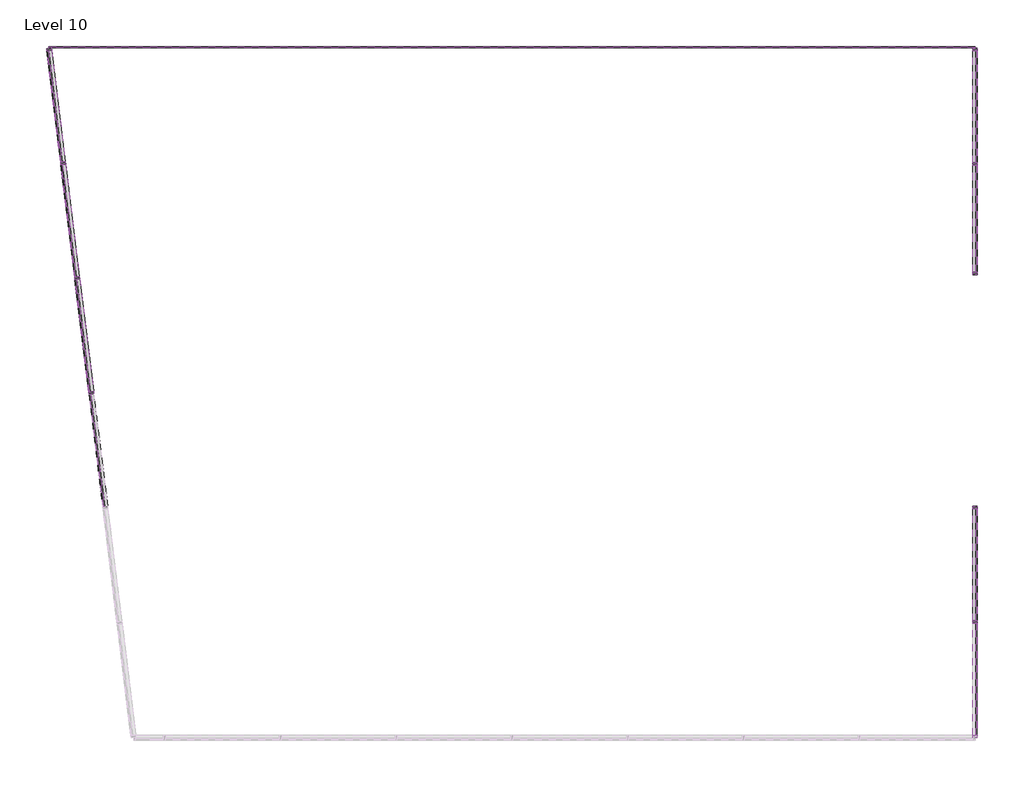
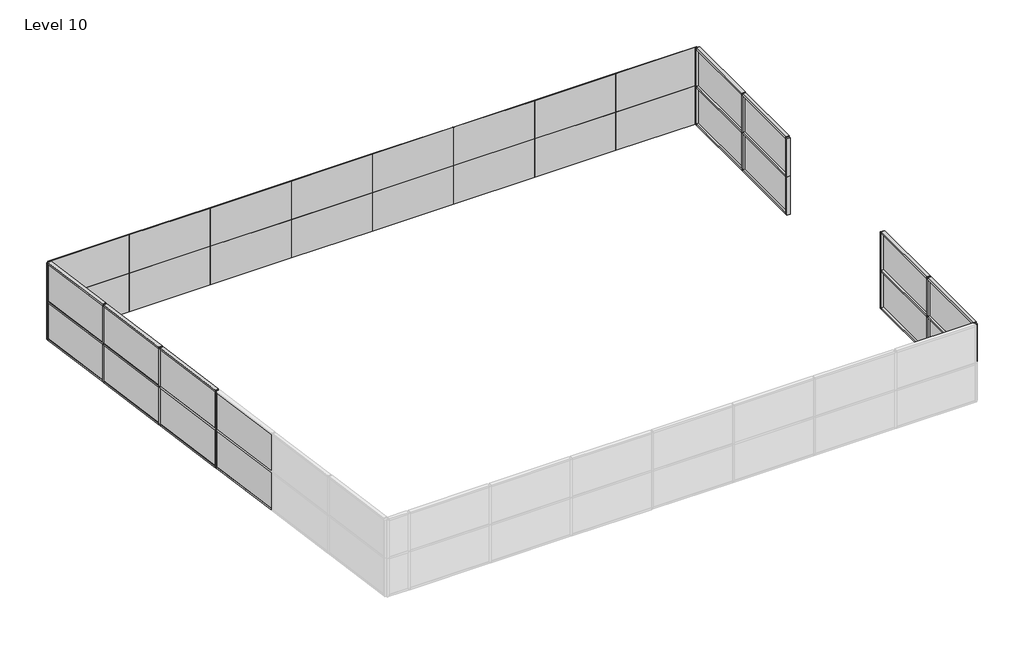
# One storey, part 2 of 2: 54 members, 40 plates.
"""IFC4 building model written with IfcOpenShell, lengths in millimetres."""

from ifc_helpers import new_model, si_unit, origin, place, context, project, spatial, transform, mapped, element, save
from components import member_71c27fd2, member_19d0a4ec, member_8cef0660, member_db480205, member_82905deb, member_4491d118, member_1b94d493, member_46bdb8c2, system_panel_glazed_1e57f9bb, system_panel_glazed_37f15d2e, system_panel_glazed_3620f98e, system_panel_glazed_e46d4b42, system_panel_glazed_2a6c68b7, system_panel_glazed_7fb1fc2b, system_panel_glazed_d483336f

model = new_model("IFC4")

# Units and contexts
model_context = context("Model", 3, world=origin())
ifc_project = project(units=[si_unit("LENGTHUNIT", "METRE", prefix="MILLI")], contexts=[model_context])

# Site, building, storey
site = spatial("IfcSite", under=ifc_project)
building = spatial("IfcBuilding", under=site)
storey = spatial("IfcBuildingStorey", under=building, Name="Level 10", Elevation=27432.0)

# Members
placement = place(None, origin())
member_shape = member_71c27fd2(model_context)
element("IfcMember", 1, ObjectType="Rectangular Mullion : 2.5\" x 5\" rectangular", at=placement, inside=storey, context=model_context, shape_type="MappedRepresentation", body=[
    mapped(member_shape, transform((-10473.7456604, 11109.5209701, 27432.0), x_axis=(0.0, 0.0, -1.0), y_axis=(-0.9925461516413222, -0.12186934340514599, 0.0), z_axis=(-0.12186934340514599, 0.9925461516413222, 0.0))),
])
element("IfcMember", 2, ObjectType="Rectangular Mullion : 2.5\" x 5\" rectangular", at=placement, inside=storey, context=model_context, shape_type="MappedRepresentation", body=[
    mapped(member_shape, transform((13902.5156363, -3899.3863708, 27432.0), x_axis=(0.0, 0.0, -1.0), y_axis=(1.0, 0.0, 0.0), z_axis=(0.0, -1.0, 0.0))),
])
element("IfcMember", 3, ObjectType="Rectangular Mullion : 2.5\" x 5\" rectangular", at=placement, inside=storey, context=model_context, shape_type="MappedRepresentation", body=[
    mapped(member_shape, transform((13902.5156363, 8156.2976505, 27432.0), x_axis=(0.0, 0.0, -1.0), y_axis=(1.0, 0.0, 0.0), z_axis=(0.0, -1.0, 0.0))),
])
member_2_shape = member_19d0a4ec(model_context)
element("IfcMember", 4, ObjectType="Rectangular Mullion : 2.5\" x 5\" rectangular", at=placement, inside=storey, context=model_context, shape_type="MappedRepresentation", body=[
    mapped(member_2_shape, transform((-10113.8959567, 8178.7803212, 28956.0), x_axis=(0.0, 0.0, 1.0), y_axis=(-0.9925461516413222, -0.12186934340514609, 0.0), z_axis=(0.12186934340514609, -0.9925461516413222, 0.0))),
])
element("IfcMember", 5, ObjectType="Rectangular Mullion : 2.5\" x 5\" rectangular", at=placement, inside=storey, context=model_context, shape_type="MappedRepresentation", body=[
    mapped(member_2_shape, transform((-10113.8959567, 8178.7803212, 30480.0), x_axis=(0.0, 0.0, 1.0), y_axis=(-0.9925461516413222, -0.12186934340514617, 0.0), z_axis=(0.12186934340514617, -0.9925461516413222, 0.0))),
])
element("IfcMember", 6, ObjectType="Rectangular Mullion : 2.5\" x 5\" rectangular", at=placement, inside=storey, context=model_context, shape_type="MappedRepresentation", body=[
    mapped(member_2_shape, transform((-10113.8959567, 8178.7803212, 28956.0), x_axis=(0.0, 0.0, 1.0), y_axis=(-0.9925461516413222, -0.12186934340514599, 0.0), z_axis=(0.12186934340514599, -0.9925461516413222, 0.0))),
])
element("IfcMember", 7, ObjectType="Rectangular Mullion : 2.5\" x 5\" rectangular", at=placement, inside=storey, context=model_context, shape_type="MappedRepresentation", body=[
    mapped(member_2_shape, transform((-10113.8959567, 8178.7803212, 30480.0), x_axis=(0.0, 0.0, 1.0), y_axis=(-0.9925461516413222, -0.12186934340514599, 0.0), z_axis=(0.12186934340514599, -0.9925461516413222, 0.0))),
])
element("IfcMember", 8, ObjectType="Rectangular Mullion : 2.5\" x 5\" rectangular", at=placement, inside=storey, context=model_context, shape_type="MappedRepresentation", body=[
    mapped(member_2_shape, transform((13902.5156363, -946.6363705, 28956.0), x_axis=(0.0, 0.0, 1.0), y_axis=(1.0, 0.0, 0.0), z_axis=(0.0, 1.0, 0.0))),
])
element("IfcMember", 9, ObjectType="Rectangular Mullion : 2.5\" x 5\" rectangular", at=placement, inside=storey, context=model_context, shape_type="MappedRepresentation", body=[
    mapped(member_2_shape, transform((13902.5156363, -3962.8863708, 28956.0), x_axis=(0.0, 0.0, 1.0), y_axis=(1.0, 0.0, 0.0), z_axis=(0.0, 1.0, 0.0))),
])
element("IfcMember", 10, ObjectType="Rectangular Mullion : 2.5\" x 5\" rectangular", at=placement, inside=storey, context=model_context, shape_type="MappedRepresentation", body=[
    mapped(member_2_shape, transform((13902.5156363, -946.6363705, 30480.0), x_axis=(0.0, 0.0, 1.0), y_axis=(1.0, 0.0, 0.0), z_axis=(0.0, 1.0, 0.0))),
])
element("IfcMember", 11, ObjectType="Rectangular Mullion : 2.5\" x 5\" rectangular", at=placement, inside=storey, context=model_context, shape_type="MappedRepresentation", body=[
    mapped(member_2_shape, transform((13902.5156363, -3962.8863708, 30480.0), x_axis=(0.0, 0.0, 1.0), y_axis=(1.0, 0.0, 0.0), z_axis=(0.0, 1.0, 0.0))),
])
element("IfcMember", 12, ObjectType="Rectangular Mullion : 2.5\" x 5\" rectangular", at=placement, inside=storey, context=model_context, shape_type="MappedRepresentation", body=[
    mapped(member_2_shape, transform((13902.5156363, 11109.0476508, 28956.0), x_axis=(0.0, 0.0, 1.0), y_axis=(1.0, 0.0, 0.0), z_axis=(0.0, 1.0, 0.0))),
])
element("IfcMember", 13, ObjectType="Rectangular Mullion : 2.5\" x 5\" rectangular", at=placement, inside=storey, context=model_context, shape_type="MappedRepresentation", body=[
    mapped(member_2_shape, transform((13902.5156363, 11109.0476508, 30480.0), x_axis=(0.0, 0.0, 1.0), y_axis=(1.0, 0.0, 0.0), z_axis=(0.0, 1.0, 0.0))),
])
member_3_shape = member_8cef0660(model_context)
element("IfcMember", 14, ObjectType="Rectangular Mullion : 2.5\" x 5\" rectangular", at=placement, inside=storey, context=model_context, shape_type="MappedRepresentation", body=[
    mapped(member_3_shape, transform((-9370.9804393, 2128.2189808, 28956.0), x_axis=(0.0, 0.0, 1.0), y_axis=(-0.9925461516413223, -0.12186934340514563, 0.0), z_axis=(0.12186934340514562, -0.9925461516413222, 0.0))),
])
element("IfcMember", 15, ObjectType="Rectangular Mullion : 2.5\" x 5\" rectangular", at=placement, inside=storey, context=model_context, shape_type="MappedRepresentation", body=[
    mapped(member_3_shape, transform((-9742.438198, 5153.499651, 28956.0), x_axis=(0.0, 0.0, 1.0), y_axis=(-0.9925461516413222, -0.12186934340514602, 0.0), z_axis=(0.12186934340514602, -0.9925461516413222, 0.0))),
])
element("IfcMember", 16, ObjectType="Rectangular Mullion : 2.5\" x 5\" rectangular", at=placement, inside=storey, context=model_context, shape_type="MappedRepresentation", body=[
    mapped(member_3_shape, transform((-9370.9804393, 2128.2189808, 30480.0), x_axis=(0.0, 0.0, 1.0), y_axis=(-0.9925461516413222, -0.12186934340514592, 0.0), z_axis=(0.12186934340514592, -0.9925461516413222, 0.0))),
])
element("IfcMember", 17, ObjectType="Rectangular Mullion : 2.5\" x 5\" rectangular", at=placement, inside=storey, context=model_context, shape_type="MappedRepresentation", body=[
    mapped(member_3_shape, transform((-9742.438198, 5153.499651, 30480.0), x_axis=(0.0, 0.0, 1.0), y_axis=(-0.9925461516413222, -0.1218693434051457, 0.0), z_axis=(0.1218693434051457, -0.9925461516413222, 0.0))),
])
element("IfcMember", 18, ObjectType="Rectangular Mullion : 2.5\" x 5\" rectangular", at=placement, inside=storey, context=model_context, shape_type="MappedRepresentation", body=[
    mapped(member_3_shape, transform((-9370.9804393, 2128.2189808, 28956.0), x_axis=(0.0, 0.0, 1.0), y_axis=(-0.9925461516413222, -0.12186934340514592, 0.0), z_axis=(0.12186934340514592, -0.9925461516413222, 0.0))),
])
element("IfcMember", 19, ObjectType="Rectangular Mullion : 2.5\" x 5\" rectangular", at=placement, inside=storey, context=model_context, shape_type="MappedRepresentation", body=[
    mapped(member_3_shape, transform((-9742.438198, 5153.499651, 28956.0), x_axis=(0.0, 0.0, 1.0), y_axis=(-0.9925461516413222, -0.1218693434051457, 0.0), z_axis=(0.1218693434051457, -0.9925461516413222, 0.0))),
])
element("IfcMember", 20, ObjectType="Rectangular Mullion : 2.5\" x 5\" rectangular", at=placement, inside=storey, context=model_context, shape_type="MappedRepresentation", body=[
    mapped(member_3_shape, transform((-9370.9804393, 2128.2189808, 30480.0), x_axis=(0.0, 0.0, 1.0), y_axis=(-0.9925461516413222, -0.12186934340514595, 0.0), z_axis=(0.12186934340514595, -0.9925461516413222, 0.0))),
])
element("IfcMember", 21, ObjectType="Rectangular Mullion : 2.5\" x 5\" rectangular", at=placement, inside=storey, context=model_context, shape_type="MappedRepresentation", body=[
    mapped(member_3_shape, transform((-9742.438198, 5153.499651, 30480.0), x_axis=(0.0, 0.0, 1.0), y_axis=(-0.9925461516413222, -0.12186934340514606, 0.0), z_axis=(0.12186934340514606, -0.9925461516413222, 0.0))),
])
member_4_shape = member_db480205(model_context)
element("IfcMember", 22, ObjectType="Rectangular Mullion : 2.5\" x 5\" rectangular", at=placement, inside=storey, context=model_context, shape_type="MappedRepresentation", body=[
    mapped(member_4_shape, transform((-9363.241736, 2065.1923001, 27432.0), x_axis=(0.0, 0.0, -1.0), y_axis=(-0.9925461516413223, -0.12186934340514559, 0.0), z_axis=(-0.12186934340514559, 0.9925461516413223, 0.0))),
])
element("IfcMember", 23, ObjectType="Rectangular Mullion : 2.5\" x 5\" rectangular", at=placement, inside=storey, context=model_context, shape_type="MappedRepresentation", body=[
    mapped(member_4_shape, transform((-9734.6994947, 5090.4729703, 27432.0), x_axis=(0.0, 0.0, -1.0), y_axis=(-0.9925461516413222, -0.12186934340514592, 0.0), z_axis=(-0.12186934340514592, 0.9925461516413222, 0.0))),
])
element("IfcMember", 24, ObjectType="Rectangular Mullion : 2.5\" x 5\" rectangular", at=placement, inside=storey, context=model_context, shape_type="MappedRepresentation", body=[
    mapped(member_4_shape, transform((-10106.1572534, 8115.7536405, 27432.0), x_axis=(0.0, 0.0, -1.0), y_axis=(-0.9925461516413222, -0.12186934340514606, 0.0), z_axis=(-0.12186934340514606, 0.9925461516413222, 0.0))),
])
member_5_shape = member_82905deb(model_context)
element("IfcMember", 25, ObjectType="Rectangular Mullion : 2.5\" x 5\" rectangular", at=placement, inside=storey, context=model_context, shape_type="MappedRepresentation", body=[
    mapped(member_5_shape, transform((-9367.1110876, 2096.7056405, 28956.0), x_axis=(-0.1218693434051459, 0.9925461516413222, 0.0), y_axis=(-0.9925461516413222, -0.1218693434051459, 0.0), z_axis=(0.0, 0.0, 1.0))),
])
element("IfcMember", 26, ObjectType="Rectangular Mullion : 2.5\" x 5\" rectangular", at=placement, inside=storey, context=model_context, shape_type="MappedRepresentation", body=[
    mapped(member_5_shape, transform((-9738.5688463, 5121.9863107, 28956.0), x_axis=(-0.1218693434051459, 0.9925461516413222, 0.0), y_axis=(-0.9925461516413222, -0.1218693434051459, 0.0), z_axis=(0.0, 0.0, 1.0))),
])
element("IfcMember", 27, ObjectType="Rectangular Mullion : 2.5\" x 5\" rectangular", at=placement, inside=storey, context=model_context, shape_type="MappedRepresentation", body=[
    mapped(member_5_shape, transform((-10110.026605, 8147.2669809, 28956.0), x_axis=(-0.1218693434051459, 0.9925461516413222, 0.0), y_axis=(-0.9925461516413222, -0.1218693434051459, 0.0), z_axis=(0.0, 0.0, 1.0))),
])
element("IfcMember", 28, ObjectType="Rectangular Mullion : 2.5\" x 5\" rectangular", at=placement, inside=storey, context=model_context, shape_type="MappedRepresentation", body=[
    mapped(member_5_shape, transform((13902.5156363, -3931.1363708, 28956.0), x_axis=(0.0, -1.0, 0.0), y_axis=(1.0, 0.0, 0.0), z_axis=(0.0, 0.0, 1.0))),
])
element("IfcMember", 29, ObjectType="Rectangular Mullion : 2.5\" x 5\" rectangular", at=placement, inside=storey, context=model_context, shape_type="MappedRepresentation", body=[
    mapped(member_5_shape, transform((13902.5156363, 8124.5476505, 28956.0), x_axis=(0.0, -1.0, 0.0), y_axis=(1.0, 0.0, 0.0), z_axis=(0.0, 0.0, 1.0))),
])
element("IfcMember", 30, ObjectType="Rectangular Mullion : 2.5\" x 5\" rectangular", at=placement, inside=storey, context=model_context, shape_type="MappedRepresentation", body=[
    mapped(member_5_shape, transform((-9367.1110876, 2096.7056405, 28956.0), x_axis=(-0.1218693434051459, 0.9925461516413222, 0.0), y_axis=(-0.9925461516413222, -0.1218693434051459, 0.0), z_axis=(0.0, 0.0, 1.0))),
])
element("IfcMember", 31, ObjectType="Rectangular Mullion : 2.5\" x 5\" rectangular", at=placement, inside=storey, context=model_context, shape_type="MappedRepresentation", body=[
    mapped(member_5_shape, transform((-9367.1110876, 2096.7056405, 30480.0), x_axis=(-0.1218693434051459, 0.9925461516413222, 0.0), y_axis=(-0.9925461516413222, -0.1218693434051459, 0.0), z_axis=(0.0, 0.0, 1.0))),
])
element("IfcMember", 32, ObjectType="Rectangular Mullion : 2.5\" x 5\" rectangular", at=placement, inside=storey, context=model_context, shape_type="MappedRepresentation", body=[
    mapped(member_5_shape, transform((-9738.5688463, 5121.9863107, 28956.0), x_axis=(-0.1218693434051459, 0.9925461516413222, 0.0), y_axis=(-0.9925461516413222, -0.1218693434051459, 0.0), z_axis=(0.0, 0.0, 1.0))),
])
element("IfcMember", 33, ObjectType="Rectangular Mullion : 2.5\" x 5\" rectangular", at=placement, inside=storey, context=model_context, shape_type="MappedRepresentation", body=[
    mapped(member_5_shape, transform((-9738.5688463, 5121.9863107, 30480.0), x_axis=(-0.1218693434051459, 0.9925461516413222, 0.0), y_axis=(-0.9925461516413222, -0.1218693434051459, 0.0), z_axis=(0.0, 0.0, 1.0))),
])
element("IfcMember", 34, ObjectType="Rectangular Mullion : 2.5\" x 5\" rectangular", at=placement, inside=storey, context=model_context, shape_type="MappedRepresentation", body=[
    mapped(member_5_shape, transform((-10110.026605, 8147.2669809, 28956.0), x_axis=(-0.1218693434051459, 0.9925461516413222, 0.0), y_axis=(-0.9925461516413222, -0.1218693434051459, 0.0), z_axis=(0.0, 0.0, 1.0))),
])
element("IfcMember", 35, ObjectType="Rectangular Mullion : 2.5\" x 5\" rectangular", at=placement, inside=storey, context=model_context, shape_type="MappedRepresentation", body=[
    mapped(member_5_shape, transform((-10110.026605, 8147.2669809, 30480.0), x_axis=(-0.1218693434051459, 0.9925461516413222, 0.0), y_axis=(-0.9925461516413222, -0.1218693434051459, 0.0), z_axis=(0.0, 0.0, 1.0))),
])
element("IfcMember", 36, ObjectType="Rectangular Mullion : 2.5\" x 5\" rectangular", at=placement, inside=storey, context=model_context, shape_type="MappedRepresentation", body=[
    mapped(member_5_shape, transform((-9367.1110876, 2096.7056405, 30480.0), x_axis=(-0.1218693434051459, 0.9925461516413222, 0.0), y_axis=(-0.9925461516413222, -0.1218693434051459, 0.0), z_axis=(0.0, 0.0, 1.0))),
])
element("IfcMember", 37, ObjectType="Rectangular Mullion : 2.5\" x 5\" rectangular", at=placement, inside=storey, context=model_context, shape_type="MappedRepresentation", body=[
    mapped(member_5_shape, transform((-9738.5688463, 5121.9863107, 30480.0), x_axis=(-0.1218693434051459, 0.9925461516413222, 0.0), y_axis=(-0.9925461516413222, -0.1218693434051459, 0.0), z_axis=(0.0, 0.0, 1.0))),
])
element("IfcMember", 38, ObjectType="Rectangular Mullion : 2.5\" x 5\" rectangular", at=placement, inside=storey, context=model_context, shape_type="MappedRepresentation", body=[
    mapped(member_5_shape, transform((-10110.026605, 8147.2669809, 30480.0), x_axis=(-0.1218693434051459, 0.9925461516413222, 0.0), y_axis=(-0.9925461516413222, -0.1218693434051459, 0.0), z_axis=(0.0, 0.0, 1.0))),
])
element("IfcMember", 39, ObjectType="Rectangular Mullion : 2.5\" x 5\" rectangular", at=placement, inside=storey, context=model_context, shape_type="MappedRepresentation", body=[
    mapped(member_5_shape, transform((13902.5156363, -3931.1363708, 30480.0), x_axis=(0.0, -1.0, 0.0), y_axis=(1.0, 0.0, 0.0), z_axis=(0.0, 0.0, 1.0))),
])
element("IfcMember", 40, ObjectType="Rectangular Mullion : 2.5\" x 5\" rectangular", at=placement, inside=storey, context=model_context, shape_type="MappedRepresentation", body=[
    mapped(member_5_shape, transform((13902.5156363, 8124.5476505, 30480.0), x_axis=(0.0, -1.0, 0.0), y_axis=(1.0, 0.0, 0.0), z_axis=(0.0, 0.0, 1.0))),
])
member_6_shape = member_4491d118(model_context)
element("IfcMember", 41, ObjectType="Rectangular Mullion : 2.5\" x 5\" rectangular", at=placement, inside=storey, context=model_context, shape_type="MappedRepresentation", body=[
    mapped(member_6_shape, transform((13902.5156363, -883.1363705, 27432.0), x_axis=(0.0, 1.0, 0.0), y_axis=(1.0, 0.0, 0.0), z_axis=(0.0, 0.0, -1.0))),
])
element("IfcMember", 42, ObjectType="Rectangular Mullion : 2.5\" x 5\" rectangular", at=placement, inside=storey, context=model_context, shape_type="MappedRepresentation", body=[
    mapped(member_6_shape, transform((13902.5156363, 11172.5476508, 27432.0), x_axis=(0.0, 1.0, 0.0), y_axis=(1.0, 0.0, 0.0), z_axis=(0.0, 0.0, -1.0))),
])
element("IfcMember", 43, ObjectType="Rectangular Mullion : 2.5\" x 5\" rectangular", at=placement, inside=storey, context=model_context, shape_type="MappedRepresentation", body=[
    mapped(member_6_shape, transform((13902.5156363, -883.1363705, 28956.0), x_axis=(0.0, 1.0, 0.0), y_axis=(1.0, 0.0, 0.0), z_axis=(0.0, 0.0, -1.0))),
])
element("IfcMember", 44, ObjectType="Rectangular Mullion : 2.5\" x 5\" rectangular", at=placement, inside=storey, context=model_context, shape_type="MappedRepresentation", body=[
    mapped(member_6_shape, transform((13902.5156363, 11172.5476508, 28956.0), x_axis=(0.0, 1.0, 0.0), y_axis=(1.0, 0.0, 0.0), z_axis=(0.0, 0.0, -1.0))),
])
element("IfcMember", 45, ObjectType="Rectangular Mullion : 2.5\" x 5\" rectangular", at=placement, inside=storey, context=model_context, shape_type="MappedRepresentation", body=[
    mapped(member_6_shape, transform((-10481.4843637, 11172.5476508, 28956.0), x_axis=(-0.1218693434051459, 0.9925461516413222, 0.0), y_axis=(-0.9925461516413222, -0.1218693434051459, 0.0), z_axis=(0.0, 0.0, 1.0))),
])
element("IfcMember", 46, ObjectType="Rectangular Mullion : 2.5\" x 5\" rectangular", at=placement, inside=storey, context=model_context, shape_type="MappedRepresentation", body=[
    mapped(member_6_shape, transform((13902.5156363, 5212.8636295, 28956.0), x_axis=(0.0, -1.0, 0.0), y_axis=(1.0, 0.0, 0.0), z_axis=(0.0, 0.0, 1.0))),
])
element("IfcMember", 47, ObjectType="Rectangular Mullion : 2.5\" x 5\" rectangular", at=placement, inside=storey, context=model_context, shape_type="MappedRepresentation", body=[
    mapped(member_6_shape, transform((-10481.4843637, 11172.5476508, 28956.0), x_axis=(-0.1218693434051459, 0.9925461516413222, 0.0), y_axis=(-0.9925461516413222, -0.1218693434051459, 0.0), z_axis=(0.0, 0.0, 1.0))),
])
element("IfcMember", 48, ObjectType="Rectangular Mullion : 2.5\" x 5\" rectangular", at=placement, inside=storey, context=model_context, shape_type="MappedRepresentation", body=[
    mapped(member_6_shape, transform((-10481.4843637, 11172.5476508, 30480.0), x_axis=(-0.1218693434051459, 0.9925461516413222, 0.0), y_axis=(-0.9925461516413222, -0.1218693434051459, 0.0), z_axis=(0.0, 0.0, 1.0))),
])
element("IfcMember", 49, ObjectType="Rectangular Mullion : 2.5\" x 5\" rectangular", at=placement, inside=storey, context=model_context, shape_type="MappedRepresentation", body=[
    mapped(member_6_shape, transform((-10481.4843637, 11172.5476508, 30480.0), x_axis=(-0.1218693434051459, 0.9925461516413222, 0.0), y_axis=(-0.9925461516413222, -0.1218693434051459, 0.0), z_axis=(0.0, 0.0, 1.0))),
])
element("IfcMember", 50, ObjectType="Rectangular Mullion : 2.5\" x 5\" rectangular", at=placement, inside=storey, context=model_context, shape_type="MappedRepresentation", body=[
    mapped(member_6_shape, transform((13902.5156363, -6979.1363705, 30480.0), x_axis=(0.0, -1.0, 0.0), y_axis=(1.0, 0.0, 0.0), z_axis=(0.0, 0.0, 1.0))),
])
element("IfcMember", 51, ObjectType="Rectangular Mullion : 2.5\" x 5\" rectangular", at=placement, inside=storey, context=model_context, shape_type="MappedRepresentation", body=[
    mapped(member_6_shape, transform((13902.5156363, 5212.8636295, 30480.0), x_axis=(0.0, -1.0, 0.0), y_axis=(1.0, 0.0, 0.0), z_axis=(0.0, 0.0, 1.0))),
])
member_7_shape = member_1b94d493(model_context)
element("IfcMember", 52, ObjectType="Rectangular Mullion : 2.5\" x 5\" rectangular", at=placement, inside=storey, context=model_context, shape_type="MappedRepresentation", body=[
    mapped(member_7_shape, transform((13902.5156363, 5276.3636295, 27432.0), x_axis=(0.0, 0.0, -1.0), y_axis=(1.0, 0.0, 0.0), z_axis=(0.0, -1.0, 0.0))),
])
member_8_shape = member_46bdb8c2(model_context)
element("IfcMember", 53, ObjectType="Rectangular Mullion : 2.5\" x 5\" rectangular", at=placement, inside=storey, context=model_context, shape_type="MappedRepresentation", body=[
    mapped(member_8_shape, transform((13902.5156363, 8092.7976505, 28956.0), x_axis=(0.0, 0.0, 1.0), y_axis=(1.0, 0.0, 0.0), z_axis=(0.0, 1.0, 0.0))),
])
element("IfcMember", 54, ObjectType="Rectangular Mullion : 2.5\" x 5\" rectangular", at=placement, inside=storey, context=model_context, shape_type="MappedRepresentation", body=[
    mapped(member_8_shape, transform((13902.5156363, 8092.7976505, 30480.0), x_axis=(0.0, 0.0, 1.0), y_axis=(1.0, 0.0, 0.0), z_axis=(0.0, 1.0, 0.0))),
])

# Plates
system_panel_glazed_shape = system_panel_glazed_1e57f9bb(model_context)
element("IfcPlate", 55, ObjectType="System Panel : Glazed", at=placement, inside=storey, context=model_context, shape_type="MappedRepresentation", body=[
    mapped(system_panel_glazed_shape, transform((-8957.4843636, 11172.5476508, 27432.0), x_axis=(1.0, 0.0, 0.0), y_axis=(0.0, 1.0, 0.0), z_axis=(0.0, 0.0, 1.0))),
])
element("IfcPlate", 56, ObjectType="System Panel : Glazed", at=placement, inside=storey, context=model_context, shape_type="MappedRepresentation", body=[
    mapped(system_panel_glazed_shape, transform((-5909.4843634, 11172.5476508, 27432.0), x_axis=(1.0, 0.0, 0.0), y_axis=(0.0, 1.0, 0.0), z_axis=(0.0, 0.0, 1.0))),
])
element("IfcPlate", 57, ObjectType="System Panel : Glazed", at=placement, inside=storey, context=model_context, shape_type="MappedRepresentation", body=[
    mapped(system_panel_glazed_shape, transform((-2861.4843634, 11172.5476508, 27432.0), x_axis=(1.0, 0.0, 0.0), y_axis=(0.0, 1.0, 0.0), z_axis=(0.0, 0.0, 1.0))),
])
element("IfcPlate", 58, ObjectType="System Panel : Glazed", at=placement, inside=storey, context=model_context, shape_type="MappedRepresentation", body=[
    mapped(system_panel_glazed_shape, transform((186.5156366, 11172.5476508, 27432.0), x_axis=(1.0, 0.0, 0.0), y_axis=(0.0, 1.0, 0.0), z_axis=(0.0, 0.0, 1.0))),
])
element("IfcPlate", 59, ObjectType="System Panel : Glazed", at=placement, inside=storey, context=model_context, shape_type="MappedRepresentation", body=[
    mapped(system_panel_glazed_shape, transform((3234.5156366, 11172.5476508, 27432.0), x_axis=(1.0, 0.0, 0.0), y_axis=(0.0, 1.0, 0.0), z_axis=(0.0, 0.0, 1.0))),
])
element("IfcPlate", 60, ObjectType="System Panel : Glazed", at=placement, inside=storey, context=model_context, shape_type="MappedRepresentation", body=[
    mapped(system_panel_glazed_shape, transform((6282.5156366, 11172.5476508, 27432.0), x_axis=(1.0, 0.0, 0.0), y_axis=(0.0, 1.0, 0.0), z_axis=(0.0, 0.0, 1.0))),
])
element("IfcPlate", 61, ObjectType="System Panel : Glazed", at=placement, inside=storey, context=model_context, shape_type="MappedRepresentation", body=[
    mapped(system_panel_glazed_shape, transform((9330.5156366, 11172.5476508, 27432.0), x_axis=(1.0, 0.0, 0.0), y_axis=(0.0, 1.0, 0.0), z_axis=(0.0, 0.0, 1.0))),
])
element("IfcPlate", 62, ObjectType="System Panel : Glazed", at=placement, inside=storey, context=model_context, shape_type="MappedRepresentation", body=[
    mapped(system_panel_glazed_shape, transform((12378.5156364, 11172.5476508, 27432.0), x_axis=(1.0, 0.0, 0.0), y_axis=(0.0, 1.0, 0.0), z_axis=(0.0, 0.0, 1.0))),
])
element("IfcPlate", 63, ObjectType="System Panel : Glazed", at=placement, inside=storey, context=model_context, shape_type="MappedRepresentation", body=[
    mapped(system_panel_glazed_shape, transform((-8957.4843636, 11172.5476508, 28956.0), x_axis=(1.0, 0.0, 0.0), y_axis=(0.0, 1.0, 0.0), z_axis=(0.0, 0.0, 1.0))),
])
element("IfcPlate", 64, ObjectType="System Panel : Glazed", at=placement, inside=storey, context=model_context, shape_type="MappedRepresentation", body=[
    mapped(system_panel_glazed_shape, transform((-5909.4843634, 11172.5476508, 28956.0), x_axis=(1.0, 0.0, 0.0), y_axis=(0.0, 1.0, 0.0), z_axis=(0.0, 0.0, 1.0))),
])
element("IfcPlate", 65, ObjectType="System Panel : Glazed", at=placement, inside=storey, context=model_context, shape_type="MappedRepresentation", body=[
    mapped(system_panel_glazed_shape, transform((-2861.4843634, 11172.5476508, 28956.0), x_axis=(1.0, 0.0, 0.0), y_axis=(0.0, 1.0, 0.0), z_axis=(0.0, 0.0, 1.0))),
])
element("IfcPlate", 66, ObjectType="System Panel : Glazed", at=placement, inside=storey, context=model_context, shape_type="MappedRepresentation", body=[
    mapped(system_panel_glazed_shape, transform((186.5156366, 11172.5476508, 28956.0), x_axis=(1.0, 0.0, 0.0), y_axis=(0.0, 1.0, 0.0), z_axis=(0.0, 0.0, 1.0))),
])
element("IfcPlate", 67, ObjectType="System Panel : Glazed", at=placement, inside=storey, context=model_context, shape_type="MappedRepresentation", body=[
    mapped(system_panel_glazed_shape, transform((3234.5156366, 11172.5476508, 28956.0), x_axis=(1.0, 0.0, 0.0), y_axis=(0.0, 1.0, 0.0), z_axis=(0.0, 0.0, 1.0))),
])
element("IfcPlate", 68, ObjectType="System Panel : Glazed", at=placement, inside=storey, context=model_context, shape_type="MappedRepresentation", body=[
    mapped(system_panel_glazed_shape, transform((6282.5156366, 11172.5476508, 28956.0), x_axis=(1.0, 0.0, 0.0), y_axis=(0.0, 1.0, 0.0), z_axis=(0.0, 0.0, 1.0))),
])
element("IfcPlate", 69, ObjectType="System Panel : Glazed", at=placement, inside=storey, context=model_context, shape_type="MappedRepresentation", body=[
    mapped(system_panel_glazed_shape, transform((9330.5156366, 11172.5476508, 28956.0), x_axis=(1.0, 0.0, 0.0), y_axis=(0.0, 1.0, 0.0), z_axis=(0.0, 0.0, 1.0))),
])
element("IfcPlate", 70, ObjectType="System Panel : Glazed", at=placement, inside=storey, context=model_context, shape_type="MappedRepresentation", body=[
    mapped(system_panel_glazed_shape, transform((12378.5156364, 11172.5476508, 28956.0), x_axis=(1.0, 0.0, 0.0), y_axis=(0.0, 1.0, 0.0), z_axis=(0.0, 0.0, 1.0))),
])
system_panel_glazed_2_shape = system_panel_glazed_37f15d2e(model_context)
element("IfcPlate", 71, ObjectType="System Panel : Glazed", at=placement, inside=storey, context=model_context, shape_type="MappedRepresentation", body=[
    mapped(system_panel_glazed_2_shape, transform((13902.5156363, -2423.0113706, 27495.5), x_axis=(0.0, -1.0, 0.0), y_axis=(1.0, 0.0, 0.0), z_axis=(0.0, 0.0, 1.0))),
])
element("IfcPlate", 72, ObjectType="System Panel : Glazed", at=placement, inside=storey, context=model_context, shape_type="MappedRepresentation", body=[
    mapped(system_panel_glazed_2_shape, transform((13902.5156363, 9632.6726506, 27495.5), x_axis=(0.0, -1.0, 0.0), y_axis=(1.0, 0.0, 0.0), z_axis=(0.0, 0.0, 1.0))),
])
element("IfcPlate", 73, ObjectType="System Panel : Glazed", at=placement, inside=storey, context=model_context, shape_type="MappedRepresentation", body=[
    mapped(system_panel_glazed_2_shape, transform((-10293.8208085, 9644.1506457, 27495.5), x_axis=(-0.1218693434051459, 0.9925461516413222, 0.0), y_axis=(-0.9925461516413222, -0.1218693434051459, 0.0), z_axis=(0.0, 0.0, 1.0))),
])
element("IfcPlate", 74, ObjectType="System Panel : Glazed", at=placement, inside=storey, context=model_context, shape_type="MappedRepresentation", body=[
    mapped(system_panel_glazed_2_shape, transform((13902.5156363, -5439.2613706, 27495.5), x_axis=(0.0, -1.0, 0.0), y_axis=(1.0, 0.0, 0.0), z_axis=(0.0, 0.0, 1.0))),
])
system_panel_glazed_3_shape = system_panel_glazed_3620f98e(model_context)
element("IfcPlate", 75, ObjectType="System Panel : Glazed", at=placement, inside=storey, context=model_context, shape_type="MappedRepresentation", body=[
    mapped(system_panel_glazed_3_shape, transform((-9181.3822083, 584.0653054, 27495.5), x_axis=(-0.1218693434051459, 0.9925461516413222, 0.0), y_axis=(-0.9925461516413222, -0.1218693434051459, 0.0), z_axis=(0.0, 0.0, 1.0))),
])
element("IfcPlate", 76, ObjectType="System Panel : Glazed", at=placement, inside=storey, context=model_context, shape_type="MappedRepresentation", body=[
    mapped(system_panel_glazed_3_shape, transform((-9552.839967, 3609.3459756, 27495.5), x_axis=(-0.1218693434051459, 0.9925461516413222, 0.0), y_axis=(-0.9925461516413222, -0.1218693434051459, 0.0), z_axis=(0.0, 0.0, 1.0))),
])
element("IfcPlate", 77, ObjectType="System Panel : Glazed", at=placement, inside=storey, context=model_context, shape_type="MappedRepresentation", body=[
    mapped(system_panel_glazed_3_shape, transform((-9924.2977257, 6634.6266458, 27495.5), x_axis=(-0.1218693434051459, 0.9925461516413222, 0.0), y_axis=(-0.9925461516413222, -0.1218693434051459, 0.0), z_axis=(0.0, 0.0, 1.0))),
])
system_panel_glazed_4_shape = system_panel_glazed_e46d4b42(model_context)
element("IfcPlate", 78, ObjectType="System Panel : Glazed", at=placement, inside=storey, context=model_context, shape_type="MappedRepresentation", body=[
    mapped(system_panel_glazed_4_shape, transform((-10293.8208085, 9644.1506457, 27463.75), x_axis=(-0.1218693434051459, 0.9925461516413222, 0.0), y_axis=(-0.9925461516413222, -0.1218693434051459, 0.0), z_axis=(0.0, 0.0, 1.0))),
])
element("IfcPlate", 79, ObjectType="System Panel : Glazed", at=placement, inside=storey, context=model_context, shape_type="MappedRepresentation", body=[
    mapped(system_panel_glazed_4_shape, transform((-10293.8208085, 9644.1506457, 28987.75), x_axis=(-0.1218693434051459, 0.9925461516413222, 0.0), y_axis=(-0.9925461516413222, -0.1218693434051459, 0.0), z_axis=(0.0, 0.0, 1.0))),
])
element("IfcPlate", 80, ObjectType="System Panel : Glazed", at=placement, inside=storey, context=model_context, shape_type="MappedRepresentation", body=[
    mapped(system_panel_glazed_4_shape, transform((-10293.8208085, 9644.1506457, 28987.75), x_axis=(-0.1218693434051459, 0.9925461516413222, 0.0), y_axis=(-0.9925461516413222, -0.1218693434051459, 0.0), z_axis=(0.0, 0.0, 1.0))),
])
element("IfcPlate", 81, ObjectType="System Panel : Glazed", at=placement, inside=storey, context=model_context, shape_type="MappedRepresentation", body=[
    mapped(system_panel_glazed_4_shape, transform((13902.5156363, -2423.0113706, 28987.75), x_axis=(0.0, -1.0, 0.0), y_axis=(1.0, 0.0, 0.0), z_axis=(0.0, 0.0, 1.0))),
])
element("IfcPlate", 82, ObjectType="System Panel : Glazed", at=placement, inside=storey, context=model_context, shape_type="MappedRepresentation", body=[
    mapped(system_panel_glazed_4_shape, transform((13902.5156363, -5439.2613706, 28987.75), x_axis=(0.0, -1.0, 0.0), y_axis=(1.0, 0.0, 0.0), z_axis=(0.0, 0.0, 1.0))),
])
element("IfcPlate", 83, ObjectType="System Panel : Glazed", at=placement, inside=storey, context=model_context, shape_type="MappedRepresentation", body=[
    mapped(system_panel_glazed_4_shape, transform((13902.5156363, 9632.6726506, 28987.75), x_axis=(0.0, -1.0, 0.0), y_axis=(1.0, 0.0, 0.0), z_axis=(0.0, 0.0, 1.0))),
])
system_panel_glazed_5_shape = system_panel_glazed_2a6c68b7(model_context)
element("IfcPlate", 84, ObjectType="System Panel : Glazed", at=placement, inside=storey, context=model_context, shape_type="MappedRepresentation", body=[
    mapped(system_panel_glazed_5_shape, transform((-9181.3822083, 584.0653054, 27463.75), x_axis=(-0.1218693434051459, 0.9925461516413222, 0.0), y_axis=(-0.9925461516413222, -0.1218693434051459, 0.0), z_axis=(0.0, 0.0, 1.0))),
])
element("IfcPlate", 85, ObjectType="System Panel : Glazed", at=placement, inside=storey, context=model_context, shape_type="MappedRepresentation", body=[
    mapped(system_panel_glazed_5_shape, transform((-9552.839967, 3609.3459756, 27463.75), x_axis=(-0.1218693434051459, 0.9925461516413222, 0.0), y_axis=(-0.9925461516413222, -0.1218693434051459, 0.0), z_axis=(0.0, 0.0, 1.0))),
])
element("IfcPlate", 86, ObjectType="System Panel : Glazed", at=placement, inside=storey, context=model_context, shape_type="MappedRepresentation", body=[
    mapped(system_panel_glazed_5_shape, transform((-9924.2977257, 6634.6266458, 27463.75), x_axis=(-0.1218693434051459, 0.9925461516413222, 0.0), y_axis=(-0.9925461516413222, -0.1218693434051459, 0.0), z_axis=(0.0, 0.0, 1.0))),
])
element("IfcPlate", 87, ObjectType="System Panel : Glazed", at=placement, inside=storey, context=model_context, shape_type="MappedRepresentation", body=[
    mapped(system_panel_glazed_5_shape, transform((-9181.3822083, 584.0653054, 28987.75), x_axis=(-0.1218693434051459, 0.9925461516413222, 0.0), y_axis=(-0.9925461516413222, -0.1218693434051459, 0.0), z_axis=(0.0, 0.0, 1.0))),
])
element("IfcPlate", 88, ObjectType="System Panel : Glazed", at=placement, inside=storey, context=model_context, shape_type="MappedRepresentation", body=[
    mapped(system_panel_glazed_5_shape, transform((-9552.839967, 3609.3459756, 28987.75), x_axis=(-0.1218693434051459, 0.9925461516413222, 0.0), y_axis=(-0.9925461516413222, -0.1218693434051459, 0.0), z_axis=(0.0, 0.0, 1.0))),
])
element("IfcPlate", 89, ObjectType="System Panel : Glazed", at=placement, inside=storey, context=model_context, shape_type="MappedRepresentation", body=[
    mapped(system_panel_glazed_5_shape, transform((-9924.2977257, 6634.6266458, 28987.75), x_axis=(-0.1218693434051459, 0.9925461516413222, 0.0), y_axis=(-0.9925461516413222, -0.1218693434051459, 0.0), z_axis=(0.0, 0.0, 1.0))),
])
element("IfcPlate", 90, ObjectType="System Panel : Glazed", at=placement, inside=storey, context=model_context, shape_type="MappedRepresentation", body=[
    mapped(system_panel_glazed_5_shape, transform((-9181.3822083, 584.0653054, 28987.75), x_axis=(-0.1218693434051459, 0.9925461516413222, 0.0), y_axis=(-0.9925461516413222, -0.1218693434051459, 0.0), z_axis=(0.0, 0.0, 1.0))),
])
element("IfcPlate", 91, ObjectType="System Panel : Glazed", at=placement, inside=storey, context=model_context, shape_type="MappedRepresentation", body=[
    mapped(system_panel_glazed_5_shape, transform((-9552.839967, 3609.3459756, 28987.75), x_axis=(-0.1218693434051459, 0.9925461516413222, 0.0), y_axis=(-0.9925461516413222, -0.1218693434051459, 0.0), z_axis=(0.0, 0.0, 1.0))),
])
element("IfcPlate", 92, ObjectType="System Panel : Glazed", at=placement, inside=storey, context=model_context, shape_type="MappedRepresentation", body=[
    mapped(system_panel_glazed_5_shape, transform((-9924.2977257, 6634.6266458, 28987.75), x_axis=(-0.1218693434051459, 0.9925461516413222, 0.0), y_axis=(-0.9925461516413222, -0.1218693434051459, 0.0), z_axis=(0.0, 0.0, 1.0))),
])
system_panel_glazed_6_shape = system_panel_glazed_7fb1fc2b(model_context)
element("IfcPlate", 93, ObjectType="System Panel : Glazed", at=placement, inside=storey, context=model_context, shape_type="MappedRepresentation", body=[
    mapped(system_panel_glazed_6_shape, transform((13902.5156363, 6684.58064, 27495.5), x_axis=(0.0, -1.0, 0.0), y_axis=(1.0, 0.0, 0.0), z_axis=(0.0, 0.0, 1.0))),
])
system_panel_glazed_7_shape = system_panel_glazed_d483336f(model_context)
element("IfcPlate", 94, ObjectType="System Panel : Glazed", at=placement, inside=storey, context=model_context, shape_type="MappedRepresentation", body=[
    mapped(system_panel_glazed_7_shape, transform((13902.5156363, 6684.58064, 28987.75), x_axis=(0.0, -1.0, 0.0), y_axis=(1.0, 0.0, 0.0), z_axis=(0.0, 0.0, 1.0))),
])

save(model, "model.ifc")

# Revit data of these elements
# Type "Rectangular Mullion : 2.5\" x 5\" rectangular"
#   built-in parameter 1007304 = 0.416667 (stored number, unit not read)
#   built-in parameter 1007301 = 0.104167 (stored number, unit not read)
#   built-in parameter 1007300 = 0.104167 (stored number, unit not read)
# Type "System Panel : Glazed"
#   Construction Type Id = "GSP4R"
#   Analytic Construction = "1/8 in Pilkington single glazing"
#   Visual Light Transmittance = 0.9
#   Solar Heat Gain Coefficient = 0.86
#   Heat Transfer Coefficient (U) = 1.18115 BTU/(h·ft²·°F)
#   Define Thermal Properties by = 1
# Elements 1, 2, 3, 4, 5, 6, 7, 8, 9, 10, 11, 12, 13, 14, 15, 16, 17, 18, 19, 20, 21, 22, 23, 24, 25, 26, 27, 28, 29, 30, 31, 32, 33, 34, 35, 36, 37, 38, 39, 40, 41, 42, 43, 44, 45, 46, 47, 48, 49, 50, 51, 52, 53, 54 (IfcMember, "Rectangular Mullion : 2.5\" x 5\" rectangular")
#   Phase Created = New Construction
#   Materials on its faces: "Aluminum"
# Elements 55, 56, 57, 58, 59, 60, 61, 62, 63, 64, 65, 66, 67, 68, 69, 70, 71, 72, 73, 74, 75, 76, 77, 78, 79, 80, 81, 82, 83, 84, 85, 86, 87, 88, 89, 90, 91, 92, 93, 94 (IfcPlate, "System Panel : Glazed")
#   Phase Created = New Construction
#   Materials on its faces: "Glass"
# Materials
#   "Aluminum": class "Metal", colour RGB 247 247 247, transparency 0, Description = "Aluminum 6061", Cost = 0
#   "Glass": class "Glass", colour RGB 0 128 192, transparency 0.75, Description = "Soda Lime Glass", Cost = 0
